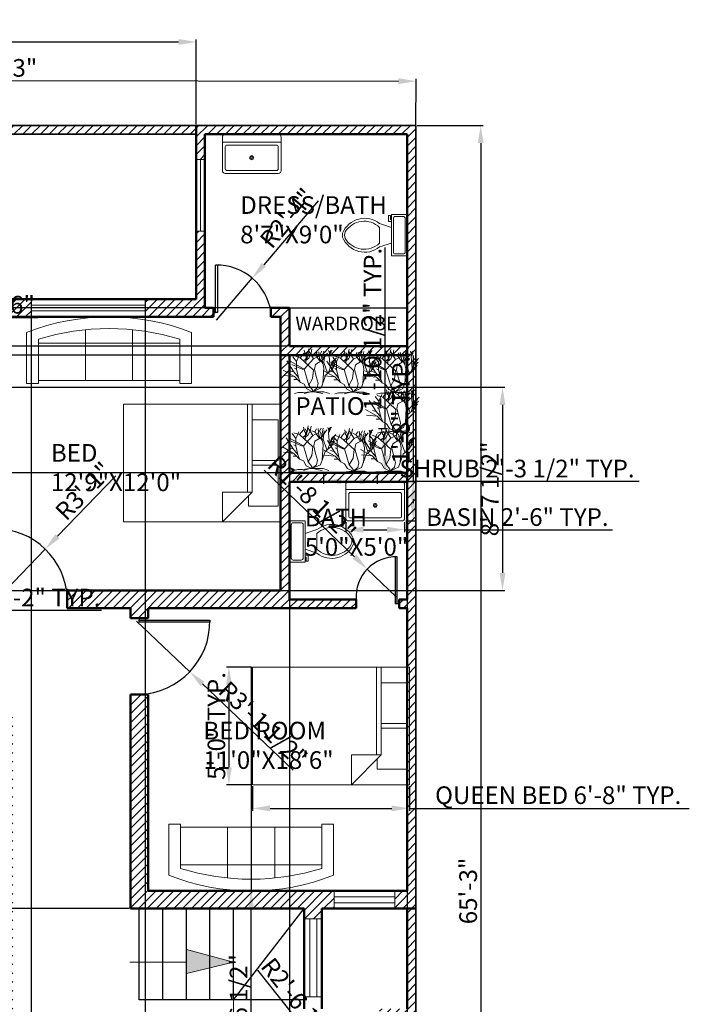
# Model space of a CAD drawing. Units: inches. Extents: x 36184 to 36805, y 18177 to 19069.
# Tile 5 of 5: x 36463 to 36805, y 18560 to 19061. Entities that reach past the tile are written whole.
import ezdxf

# ---------------------------------------------------------------- set-up
doc = ezdxf.new("R2010")
doc.units = ezdxf.units.IN
doc.linetypes.add('ACAD_ISO02W100', pattern=[15, 12, -3])
for name, color, linetype, lineweight in [('A-ANNO-DIMS', 2, 'Continuous', 18), ('A-ANNO-SYMB', 7, 'Continuous', 18), ('A-ANNO-SYMB-PATT', 7, 'Continuous', 13), ('A-AREA-IDEN', 7, 'Continuous', 25), ('A-DOOR', 4, 'Continuous', 25), ('A-FLOR-CASE', 9, 'Continuous', 25), ('A-FLOR-FIXT', 9, 'Continuous', 18), ('A-FLOR-STRS', 7, 'Continuous', 25), ('A-FLOR-STRS-OVHD', 7, 'ACAD_ISO02W100', 18), ('A-FURN', 8, 'Continuous', 18), ('A-GLAZ', 4, 'Continuous', 18), ('A-WALL', 7, 'Continuous', 50), ('C-PROP', 7, 'Continuous', 35), ('L-PLNT', 94, 'Continuous', 13), ('L-SITE-WALL', 7, 'Continuous', 35)]:
    doc.layers.add(name, color=color, linetype=linetype, lineweight=lineweight)
doc.layers.add('A-WALL-PATT', color=244, linetype='Continuous', lineweight=13, true_color=0x991b1e)
doc.styles.get("Standard").update_dxf_attribs({"font": 'arial.ttf'})
doc.dimstyles.new('ISO-25', dxfattribs={"dimtxt": 9, "dimasz": 9, "dimexe": 1.25, "dimexo": 0.625, "dimtad": 1, "dimdec": 1, "dimrnd": 9, "dimlunit": 3, "dimtxsty": 'Standard', "dimcen": 2.5, "dimadec": 0, "dimazin": 0, "dimtfac": 1, "dimtdec": 1, "dimtmove": 0, "dimatfit": 3, "dimfxl": 1, "dimarcsym": 0})

# ---------------------------------------------------------------- blocks, each defined once
blk = doc.blocks.new('Sofa - Roundback 7 ft.')
for p, q in [((-12.00002, -32.4421), (-12.00003, -6.5971)), ((11.99997, -32.4421), (11.99998, -6.5971)), ((-36.000027, -34), (-36.000027, -11.4696)), ((-35.999844, -13.3819), (35.9998, -13.3819)), ((35.99998, -34), (35.99998, -11.4696)), ((-36.000027, -32.4421), (35.99998, -32.4421))]:
    blk.add_line(p, q)
for points in [[(-36.000027, -34), (-42.000027, -34), (-42.000027, -8)], [(41.99998, -8), (41.99998, -34), (35.99998, -34)]]:
    blk.add_lwpolyline(points)
for centre, radius, start, end in [((0, -114.25), 114.25, 68.43141, 111.5686), ((-0.00001, -127.1968), 121.1968, 72.72033, 107.2797)]:
    blk.add_arc(centre, radius, start, end)
blk = doc.blocks.new('Bed - Queen')
for p, q in [((0, -80.00003), (0, 0)), ((0, 0), (59.99999, 0)), ((59.99999, 0), (59.99999, -80.00003)), ((7.99999, -1.2), (28.79998, -1.2)), ((7.99999, -14.4), (7.99999, -1.2)), ((28.79998, -1.2), (28.79998, -14.4)), ((31.19999, -1.2), (51.99999, -1.2)), ((31.19999, -14.4), (31.19999, -1.2)), ((51.99999, -1.2), (51.99999, -16.4)), ((0, -14.4), (44.8, -14.4)), ((59.99999, -29.6), (44.8, -14.4)), ((44.8, -14.4), (44.8, -29.6)), ((44.8, -16.8), (0, -16.8)), ((51.99999, -16.4), (46.79936, -16.4)), ((44.8, -29.6), (59.99999, -29.6)), ((59.99999, -80.00003), (0, -80.00003))]:
    blk.add_line(p, q)
blk = doc.blocks.new('Toilet - top')
for p, q in [((9.5, -6), (9.5, -2)), ((-10, -8.5), (-8, -8.5)), ((-10, -9.5), (-10, -8.5)), ((-7, -9.5), (-10, -9.5)), ((-8, -8.5), (-8, -8)), ((-7, -8), (-7, -9.5)), ((-4, -8), (-6, -14)), ((4, -8), (6, -14)), ((4, -14), (-4, -14))]:
    blk.add_line(p, q)
blk.add_lwpolyline([(10.5, -8), (10.5, 0), (-10.5, 0), (-10.5, -8)], close=True)
for points in [[(-9.5, -2), (-9.5, -6)], [(8.5, -1), (-8.5, -1)], [(-8.5, -7), (8.5, -7)]]:
    blk.add_lwpolyline(points)
for centre, radius, start, end in [((-8.62, -1.88), 0.884, 81.8699, 188.1301), ((8.62, -1.88), 0.884, 351.8699, 98.1301), ((-8.62, -6.12), 0.884, 171.8699, 278.1301), ((8.62, -6.12), 0.884, 261.8699, 8.1301), ((3.52, -21.58), 12.17, 141.4691, 247.9714), ((4.2, -21.82), 11.33, 136.3677, 238.9468), ((-3.52, -21.58), 12.17, 292.0284, 38.5307), ((-4.2, -21.82), 11.33, 301.053, 43.6321), ((0, -27.88), 4, 245.7318, 294.2682), ((0, -29), 4, 254.8605, 285.1395)]:
    blk.add_arc(centre, radius, start, end)
blk = doc.blocks.new('Sink-single - 30 in top')
blk.add_line((-15, -3.999996), (15, -3.999996))
for points in [[(-13.5, 0), (13.5, 0)], [(-15, -18.499996), (-15, -1.5)], [(15, -1.5), (15, -18.499996)], [(-13.5, -17.499996), (-13.5, -6.499996)], [(-12.5, -5.499996), (12.5, -5.499996)], [(13.5, -6.499996), (13.5, -17.499996)], [(13.5, -19.999996), (-13.5, -19.999996)], [(12.5, -18.499996), (-12.5, -18.499996)]]:
    blk.add_lwpolyline(points)
for radius in [1, 0.5]:
    blk.add_circle((0, -11.999996), radius)
for centre, radius, start, end in [((-13.5, -1.5), 1.5, 90, 180), ((13.5, -1.5), 1.5, 0, 90), ((-12.5, -6.499996), 1, 90, 180), ((12.5, -6.499996), 1, 0, 90), ((-13.5, -18.499996), 1.5, 180, 270), ((-12.5, -17.499996), 1, 180, 270), ((12.5, -17.499996), 1, 270, 0), ((13.5, -18.499996), 1.5, 270, 0)]:
    blk.add_arc(centre, radius, start, end)
blk = doc.blocks.new('*D13')
at = {"layer": 'A-ANNO-DIMS', "color": 0, "lineweight": -2, "transparency": 16777216}
for p, q in [((36245.31, 19007.93), (36245.36, 19031.89)), ((36665.31, 19007.11), (36665.36, 19031.07)), ((36254.36, 19030.62), (36656.36, 19029.84))]:
    blk.add_line(p, q, dxfattribs=at)
at = {"layer": 'A-ANNO-DIMS', "color": 0, "transparency": 16777216}
for points in [[(36254.36, 19032.12), (36254.35, 19029.12), (36245.36, 19030.64)], [(36656.36, 19031.34), (36656.35, 19028.34), (36665.36, 19029.82)]]:
    blk.add_solid(points, dxfattribs=at)
at = {"layer": 'Defpoints', "color": 0, "transparency": 16777216}
for p in [(36665.36, 19029.82), (36245.31, 19007.3), (36665.31, 19006.48)]:
    blk.add_point(p, dxfattribs=at)
at = {"layer": 'A-ANNO-DIMS', "color": 0, "transparency": 16777216, "insert": (36455.37, 19035.45), "char_height": 9, "attachment_point": 5, "rotation": 359.8885}
blk.add_mtext('35\'-3"', dxfattribs=at)
blk = doc.blocks.new('*D15')
at = {"layer": 'A-ANNO-DIMS', "color": 0, "lineweight": -2, "transparency": 16777216}
for p, q in [((36665.94, 19007.3), (36699.58, 19007.3)), ((36698.33, 18998.3), (36698.33, 18236.3)), ((36665.94, 18227.3), (36699.58, 18227.3))]:
    blk.add_line(p, q, dxfattribs=at)
at = {"layer": 'A-ANNO-DIMS', "color": 0, "transparency": 16777216}
for points in [[(36696.83, 18998.3), (36699.83, 18998.3), (36698.33, 19007.3)], [(36696.83, 18236.3), (36699.83, 18236.3), (36698.33, 18227.3)]]:
    blk.add_solid(points, dxfattribs=at)
at = {"layer": 'Defpoints', "color": 0, "transparency": 16777216}
for p in [(36665.31, 19007.3), (36665.31, 18227.3), (36698.33, 18227.3)]:
    blk.add_point(p, dxfattribs=at)
at = {"layer": 'A-ANNO-DIMS', "color": 0, "transparency": 16777216, "insert": (36693.1, 18617.3), "char_height": 9, "attachment_point": 5, "rotation": 90}
blk.add_mtext('65\'-3"', dxfattribs=at)
blk = doc.blocks.new('Shrub - elevation')
for p, q in [((-14.88, 18.24), (-12.96, 20.64)), ((-12.471, 19.775), (-12.898, 22.044)), ((-11.28, 19.619), (-12.104, 21.184)), ((-11.921, 18.836), (-10.64, 20.401)), ((-11.433, 18.289), (-10.457, 22.749)), ((-8.16, 17.76), (-10.56, 21.6)), ((-9.48, 19.775), (-8.992, 22.592)), ((-7.2, 19.68), (-8.64, 20.16)), ((-7.2, 19.68), (-6.24, 21.12)), ((-5.086, 17.741), (-5.513, 21.34)), ((-5.28, 19.2), (-3.84, 21.6)), ((-3.84, 16.8), (-0.96, 20.64)), ((-3.377, 18.602), (-2.888, 21.575)), ((-2.88, 15.84), (-2.4, 20.16)), ((-0.508, 21.888), (-0.081, 20.558)), ((-0.203, 19.149), (0.102, 21.34)), ((-0.142, 19.384), (0.59, 20.401)), ((-0.02, 20.01), (0.896, 21.105)), ((0.041, 20.714), (1.384, 22.044)), ((0.102, 21.34), (0.835, 21.888)), ((-18.24, 11.04), (-21.755, 16.655)), ((-12.96, 12.48), (-19.68, 16.32)), ((-16.8, 16.32), (-18.72, 18.72)), ((-14.88, 18.24), (-17.76, 19.2)), ((-16.8, 16.32), (-15.36, 19.68)), ((-16.8, 12.48), (-16.8, 16.32)), ((-8.16, 12), (-14.88, 18.24)), ((-13.325, 16.724), (-11.433, 18.289)), ((-12.96, 12.48), (-8.16, 17.76)), ((-11.677, 19.071), (-12.471, 19.775)), ((-12.043, 15.628), (-11.921, 18.836)), ((-11.982, 16.802), (-10.579, 18.054)), ((-10.579, 18.054), (-9.846, 19.697)), ((-8.16, 17.76), (-5.28, 19.2)), ((-4.8, 16.32), (-7.2, 19.68)), ((-7.2, 14.88), (-3.84, 16.8)), ((-3.377, 15.315), (-5.086, 17.819)), ((-2.88, 12.96), (-4.32, 19.68)), ((-2.766, 16.802), (-3.377, 18.602)), ((-0.96, 10.56), (-2.88, 15.84)), ((0.346, 13.203), (-0.203, 19.149)), ((0.346, 13.203), (1.323, 16.254)), ((0.96, 12), (1.44, 15.36)), ((1.323, 16.254), (3.642, 18.289)), ((1.44, 15.36), (2.88, 17.28)), ((1.92, 13.44), (2.4, 15.36)), ((2.4, 15.36), (3.36, 16.32)), ((-17.76, 8.64), (-23.663, 11.961)), ((-18.24, 11.04), (-20.16, 11.52)), ((-13.92, 12.48), (-19.2, 14.88)), ((-15.84, 8.16), (-18.24, 11.04)), ((-16.8, 12.48), (-17.76, 12.96)), ((-15.84, 8.16), (-16.8, 12.48)), ((-12.96, 12.48), (-13.92, 12.48)), ((-10.56, 4.32), (-12.96, 12.48)), ((-8.64, 7.68), (-8.16, 12)), ((-7.68, 12.48), (-7.2, 14.88)), ((-6.72, 8.64), (-7.68, 12.48)), ((-3.36, 5.28), (-2.88, 12.96)), ((-1.92, 9.6), (0.96, 12)), ((-0.48, 10.8), (0.346, 13.203)), ((0.96, 12), (2.88, 14.88)), ((-17.76, 8.64), (-23.128, 9.222)), ((-16.32, 7.2), (-18.24, 7.2)), ((-14.88, 5.76), (-17.76, 8.64)), ((-14.88, 5.76), (-15.84, 8.16)), ((-12.96, 4.8), (-14.88, 5.76)), ((-10.56, 4.32), (-8.64, 7.68)), ((-5.76, 5.28), (-6.72, 8.64)), ((-6.24, 2.88), (-5.76, 5.28)), ((-4.32, 2.88), (-1.92, 9.6)), ((-15.84, 0.48), (-17.76, 0)), ((-13.44, 0.48), (-15.84, 0.48)), ((-9.6, 0.96), (-13.44, 0.48)), ((-11.52, 2.4), (-12.96, 4.8)), ((-9.6, 0.96), (-12.96, 0)), ((-8.64, 0.96), (-11.52, 2.4)), ((-8.64, 1.92), (-10.56, 4.32)), ((-9.6, 0.96), (-7.68, 0.96)), ((-8.64, 0.96), (-4.32, 2.88)), ((-8.64, 0.96), (-6.24, 2.88)), ((-8.64, 0.96), (-8.64, 1.92)), ((-8.64, 0.96), (-2.88, 0.96)), ((-7.68, 0.96), (-6.24, 0.48)), ((-6.24, 0.48), (-3.36, 0)), ((-2.88, 0.96), (0, 0))]:
    blk.add_line(p, q)
blk = doc.blocks.new('DOOR-LEAF-24IN')
for p, q in [((1, 0), (1, 24)), ((1, 24), (2, 24)), ((2, 24), (2, 0)), ((0, 0), (1, 0)), ((1, 0), (2, 0))]:
    blk.add_line(p, q)
blk = doc.blocks.new('DOOR-LEAF-36IN')
for p, q in [((1, 36), (0, 36)), ((0, 36), (0, 0)), ((1, 0), (1, 36)), ((0, 0), (1, 0)), ((2, 0), (1, 0))]:
    blk.add_line(p, q)
blk = doc.blocks.new('*D24')
at = {"layer": 'A-ANNO-DIMS', "color": 0, "lineweight": -2, "transparency": 16777216}
for p, q in [((36618.26, 18829.49), (36618.26, 18824.77)), ((36627.26, 18826.02), (36636.57, 18826.02)), ((36645.57, 18829.49), (36645.57, 18824.77)), ((36645.57, 18826.02), (36779.11, 18826.02))]:
    blk.add_line(p, q, dxfattribs=at)
at = {"layer": 'A-ANNO-DIMS', "color": 0, "transparency": 16777216}
for points in [[(36627.26, 18827.52), (36627.26, 18824.52), (36618.26, 18826.02)], [(36636.57, 18827.52), (36636.57, 18824.52), (36645.57, 18826.02)]]:
    blk.add_solid(points, dxfattribs=at)
at = {"layer": 'Defpoints', "color": 0, "transparency": 16777216}
for p in [(36618.26, 18830.12), (36645.57, 18830.12), (36645.57, 18826.02)]:
    blk.add_point(p, dxfattribs=at)
at = {"layer": 'A-ANNO-DIMS', "color": 0, "transparency": 16777216, "insert": (36716.84, 18831.31), "char_height": 9, "attachment_point": 5}
blk.add_mtext('SHRUB 2\'-3 1/2" TYP.', dxfattribs=at)
blk = doc.blocks.new('*D25')
at = {"layer": 'A-ANNO-DIMS', "color": 0, "lineweight": -2, "transparency": 16777216}
for p, q in [((36649.66, 18852.87), (36649.66, 18945.1)), ((36646.19, 18852.87), (36650.91, 18852.87)), ((36649.66, 18839.12), (36649.66, 18843.87)), ((36646.19, 18830.12), (36650.91, 18830.12))]:
    blk.add_line(p, q, dxfattribs=at)
at = {"layer": 'A-ANNO-DIMS', "color": 0, "transparency": 16777216}
for points in [[(36648.16, 18843.87), (36651.16, 18843.87), (36649.66, 18852.87)], [(36648.16, 18839.12), (36651.16, 18839.12), (36649.66, 18830.12)]]:
    blk.add_solid(points, dxfattribs=at)
at = {"layer": 'Defpoints', "color": 0, "transparency": 16777216}
for p in [(36645.57, 18852.87), (36649.66, 18852.87), (36645.57, 18830.12)]:
    blk.add_point(p, dxfattribs=at)
at = {"layer": 'A-ANNO-DIMS', "color": 0, "transparency": 16777216, "insert": (36644.38, 18903.48), "char_height": 9, "attachment_point": 5, "rotation": 90}
blk.add_mtext('1\'-10 1/2" TYP.', dxfattribs=at)
blk = doc.blocks.new('*D29')
at = {"layer": 'A-ANNO-DIMS', "color": 0, "lineweight": -2, "transparency": 16777216}
for p, q in [((36429, 18765.18), (36429, 18759.15)), ((36431, 18765.18), (36431, 18759.15)), ((36420, 18760.4), (36411, 18760.4)), ((36429, 18760.4), (36431, 18760.4)), ((36440, 18760.4), (36505.11, 18760.4))]:
    blk.add_line(p, q, dxfattribs=at)
at = {"layer": 'A-ANNO-DIMS', "color": 0, "transparency": 16777216}
for points in [[(36420, 18761.9), (36420, 18758.9), (36429, 18760.4)], [(36440, 18761.9), (36440, 18758.9), (36431, 18760.4)]]:
    blk.add_solid(points, dxfattribs=at)
at = {"layer": 'Defpoints', "color": 0, "transparency": 16777216}
for p in [(36429, 18765.8), (36431, 18765.8), (36431, 18760.4)]:
    blk.add_point(p, dxfattribs=at)
at = {"layer": 'A-ANNO-DIMS', "color": 0, "transparency": 16777216, "insert": (36477.06, 18765.62), "char_height": 9, "attachment_point": 5}
blk.add_mtext('0\'-2" TYP.', dxfattribs=at)
blk = doc.blocks.new('*D30')
at = {"layer": 'A-ANNO-DIMS', "color": 0, "lineweight": -2, "transparency": 16777216}
for p, q in [((36582.01, 18670.73), (36582.01, 18658.11)), ((36662.01, 18670.73), (36662.01, 18658.11)), ((36591.01, 18659.36), (36653.01, 18659.36)), ((36662.01, 18659.36), (36804.65, 18659.36))]:
    blk.add_line(p, q, dxfattribs=at)
at = {"layer": 'A-ANNO-DIMS', "color": 0, "transparency": 16777216}
for points in [[(36591.01, 18660.86), (36591.01, 18657.86), (36582.01, 18659.36)], [(36653.01, 18660.86), (36653.01, 18657.86), (36662.01, 18659.36)]]:
    blk.add_solid(points, dxfattribs=at)
at = {"layer": 'Defpoints', "color": 0, "transparency": 16777216}
for p in [(36582.01, 18671.36), (36662.01, 18671.36), (36662.01, 18659.36)]:
    blk.add_point(p, dxfattribs=at)
at = {"layer": 'A-ANNO-DIMS', "color": 0, "transparency": 16777216, "insert": (36737.83, 18664.91), "char_height": 9, "attachment_point": 5}
blk.add_mtext('QUEEN BED 6\'-8" TYP.', dxfattribs=at)
blk = doc.blocks.new('*D31')
at = {"layer": 'A-ANNO-DIMS', "color": 0, "lineweight": -2, "transparency": 16777216}
for p, q in [((36581.39, 18731.36), (36568.76, 18731.36)), ((36570.01, 18722.36), (36570.01, 18680.36)), ((36581.39, 18671.36), (36568.76, 18671.36))]:
    blk.add_line(p, q, dxfattribs=at)
at = {"layer": 'A-ANNO-DIMS', "color": 0, "transparency": 16777216}
for points in [[(36568.51, 18722.36), (36571.51, 18722.36), (36570.01, 18731.36)], [(36568.51, 18680.36), (36571.51, 18680.36), (36570.01, 18671.36)]]:
    blk.add_solid(points, dxfattribs=at)
at = {"layer": 'Defpoints', "color": 0, "transparency": 16777216}
for p in [(36582.01, 18731.36), (36570.01, 18671.36), (36582.01, 18671.36)]:
    blk.add_point(p, dxfattribs=at)
at = {"layer": 'A-ANNO-DIMS', "color": 0, "transparency": 16777216, "insert": (36564.79, 18701.36), "char_height": 9, "attachment_point": 5, "rotation": 90}
blk.add_mtext('5\'-0" TYP.', dxfattribs=at)
blk = doc.blocks.new('*D34')
at = {"layer": 'A-ANNO-DIMS', "color": 0, "lineweight": -2, "transparency": 16777216}
for p, q in [((36629.54, 18805.19), (36629.54, 18800.07)), ((36659.54, 18805.19), (36659.54, 18800.07)), ((36638.54, 18801.32), (36650.54, 18801.32)), ((36659.54, 18801.32), (36765.47, 18801.32))]:
    blk.add_line(p, q, dxfattribs=at)
at = {"layer": 'A-ANNO-DIMS', "color": 0, "transparency": 16777216}
for points in [[(36638.54, 18802.82), (36638.54, 18799.82), (36629.54, 18801.32)], [(36650.54, 18802.82), (36650.54, 18799.82), (36659.54, 18801.32)]]:
    blk.add_solid(points, dxfattribs=at)
at = {"layer": 'Defpoints', "color": 0, "transparency": 16777216}
for p in [(36629.54, 18805.82), (36659.54, 18805.82), (36659.54, 18801.32)]:
    blk.add_point(p, dxfattribs=at)
at = {"layer": 'A-ANNO-DIMS', "color": 0, "transparency": 16777216, "insert": (36717, 18806.6), "char_height": 9, "attachment_point": 5}
blk.add_mtext('BASIN 2\'-6" TYP.', dxfattribs=at)
blk = doc.blocks.new('*D35')
at = {"layer": 'A-ANNO-DIMS', "color": 0, "lineweight": -2, "transparency": 16777216}
for p, q in [((36664.04, 18825.82), (36664.04, 18890.08)), ((36660.16, 18825.82), (36665.29, 18825.82)), ((36664.04, 18814.82), (36664.04, 18816.82)), ((36660.16, 18805.82), (36665.29, 18805.82))]:
    blk.add_line(p, q, dxfattribs=at)
at = {"layer": 'A-ANNO-DIMS', "color": 0, "transparency": 16777216}
for points in [[(36662.54, 18816.82), (36665.54, 18816.82), (36664.04, 18825.82)], [(36662.54, 18814.82), (36665.54, 18814.82), (36664.04, 18805.82)]]:
    blk.add_solid(points, dxfattribs=at)
at = {"layer": 'Defpoints', "color": 0, "transparency": 16777216}
for p in [(36659.54, 18825.82), (36664.04, 18825.82), (36659.54, 18805.82)]:
    blk.add_point(p, dxfattribs=at)
at = {"layer": 'A-ANNO-DIMS', "color": 0, "transparency": 16777216, "insert": (36658.82, 18862.45), "char_height": 9, "attachment_point": 5, "rotation": 90}
blk.add_mtext('1\'-8" TYP.', dxfattribs=at)
blk = doc.blocks.new('*D40')
at = {"layer": 'A-ANNO-DIMS', "color": 0, "lineweight": -2, "transparency": 16777216}
for p, q in [((36360.76, 18905.62), (36360.76, 18910.74)), ((36390.76, 18905.62), (36390.76, 18910.74)), ((36369.76, 18909.49), (36381.76, 18909.49)), ((36390.76, 18909.49), (36472.67, 18909.49))]:
    blk.add_line(p, q, dxfattribs=at)
at = {"layer": 'A-ANNO-DIMS', "color": 0, "transparency": 16777216}
for points in [[(36369.76, 18910.99), (36369.76, 18907.99), (36360.76, 18909.49)], [(36381.76, 18910.99), (36381.76, 18907.99), (36390.76, 18909.49)]]:
    blk.add_solid(points, dxfattribs=at)
at = {"layer": 'Defpoints', "color": 0, "transparency": 16777216}
for p in [(36390.76, 18909.49), (36360.76, 18904.99), (36390.76, 18904.99)]:
    blk.add_point(p, dxfattribs=at)
at = {"layer": 'A-ANNO-DIMS', "color": 0, "transparency": 16777216, "insert": (36436.22, 18914.77), "char_height": 9, "attachment_point": 5}
blk.add_mtext('RANGE 2\'-6"', dxfattribs=at)
blk = doc.blocks.new('*D45')
at = {"layer": 'A-ANNO-DIMS', "color": 0, "lineweight": -2, "transparency": 16777216}
for p, q in [((36245.31, 19007.93), (36245.31, 19051.05)), ((36553.31, 19007.93), (36553.31, 19051.05)), ((36254.31, 19049.8), (36544.31, 19049.8))]:
    blk.add_line(p, q, dxfattribs=at)
at = {"layer": 'A-ANNO-DIMS', "color": 0, "transparency": 16777216}
for points in [[(36254.31, 19051.3), (36254.31, 19048.3), (36245.31, 19049.8)], [(36544.31, 19051.3), (36544.31, 19048.3), (36553.31, 19049.8)]]:
    blk.add_solid(points, dxfattribs=at)
at = {"layer": 'Defpoints', "color": 0, "transparency": 16777216}
for p in [(36553.31, 19049.8), (36245.31, 19007.3), (36553.31, 19007.3)]:
    blk.add_point(p, dxfattribs=at)
at = {"layer": 'A-ANNO-DIMS', "color": 0, "transparency": 16777216, "insert": (36399.31, 19055.02), "char_height": 9, "attachment_point": 5}
blk.add_mtext('25\'-8"', dxfattribs=at)
blk = doc.blocks.new('*D47')
at = {"layer": 'A-ANNO-DIMS', "color": 0, "lineweight": -2, "transparency": 16777216}
for p, q in [((36519.19, 18608.3), (36201.56, 18608.3)), ((36202.81, 18518.3), (36202.81, 18599.3)), ((36519.19, 18509.3), (36201.56, 18509.3))]:
    blk.add_line(p, q, dxfattribs=at)
at = {"layer": 'A-ANNO-DIMS', "color": 0, "transparency": 16777216}
for points in [[(36201.31, 18599.3), (36204.31, 18599.3), (36202.81, 18608.3)], [(36201.31, 18518.3), (36204.31, 18518.3), (36202.81, 18509.3)]]:
    blk.add_solid(points, dxfattribs=at)
at = {"layer": 'Defpoints', "color": 0, "transparency": 16777216}
for p in [(36202.81, 18608.3), (36519.81, 18608.3), (36519.81, 18509.3)]:
    blk.add_point(p, dxfattribs=at)
at = {"layer": 'A-ANNO-DIMS', "color": 0, "transparency": 16777216, "insert": (36197.59, 18558.8), "char_height": 9, "attachment_point": 5, "rotation": 90}
blk.add_mtext('8\'-3"', dxfattribs=at)
blk = doc.blocks.new('*D48')
at = {"layer": 'A-ANNO-DIMS', "color": 0, "lineweight": -2, "transparency": 16777216}
for p, q in [((36600.81, 18829.68), (36600.81, 18183.55)), ((36660.81, 18829.68), (36660.81, 18183.55)), ((36609.81, 18184.8), (36651.81, 18184.8))]:
    blk.add_line(p, q, dxfattribs=at)
at = {"layer": 'A-ANNO-DIMS', "color": 0, "transparency": 16777216}
for points in [[(36609.81, 18186.3), (36609.81, 18183.3), (36600.81, 18184.8)], [(36651.81, 18186.3), (36651.81, 18183.3), (36660.81, 18184.8)]]:
    blk.add_solid(points, dxfattribs=at)
at = {"layer": 'Defpoints', "color": 0, "transparency": 16777216}
for p in [(36600.81, 18830.3), (36660.81, 18830.3), (36660.81, 18184.8)]:
    blk.add_point(p, dxfattribs=at)
at = {"layer": 'A-ANNO-DIMS', "color": 0, "transparency": 16777216, "insert": (36630.81, 18190.02), "char_height": 9, "attachment_point": 5}
blk.add_mtext('5\'-0"', dxfattribs=at)
blk = doc.blocks.new('*D49')
at = {"layer": 'A-ANNO-DIMS', "color": 0, "lineweight": -2, "transparency": 16777216}
for p, q in [((36600.19, 18890.3), (36201.56, 18890.3)), ((36202.81, 18839.3), (36202.81, 18881.3)), ((36600.19, 18830.3), (36201.56, 18830.3))]:
    blk.add_line(p, q, dxfattribs=at)
at = {"layer": 'A-ANNO-DIMS', "color": 0, "transparency": 16777216}
for points in [[(36201.31, 18881.3), (36204.31, 18881.3), (36202.81, 18890.3)], [(36201.31, 18839.3), (36204.31, 18839.3), (36202.81, 18830.3)]]:
    blk.add_solid(points, dxfattribs=at)
at = {"layer": 'Defpoints', "color": 0, "transparency": 16777216}
for p in [(36202.81, 18890.3), (36600.81, 18890.3), (36600.81, 18830.3)]:
    blk.add_point(p, dxfattribs=at)
at = {"layer": 'A-ANNO-DIMS', "color": 0, "transparency": 16777216, "insert": (36197.59, 18860.3), "char_height": 9, "attachment_point": 5, "rotation": 90}
blk.add_mtext('5\'-0"', dxfattribs=at)
blk = doc.blocks.new('*D50')
at = {"layer": 'A-ANNO-DIMS', "color": 0, "lineweight": -2, "transparency": 16777216}
for p, q in [((36202.81, 18914.3), (36202.81, 18968.6)), ((36600.19, 18914.3), (36201.56, 18914.3)), ((36202.81, 18903.8), (36202.81, 18905.3)), ((36600.19, 18894.8), (36201.56, 18894.8))]:
    blk.add_line(p, q, dxfattribs=at)
at = {"layer": 'A-ANNO-DIMS', "color": 0, "transparency": 16777216}
for points in [[(36201.31, 18905.3), (36204.31, 18905.3), (36202.81, 18914.3)], [(36201.31, 18903.8), (36204.31, 18903.8), (36202.81, 18894.8)]]:
    blk.add_solid(points, dxfattribs=at)
at = {"layer": 'Defpoints', "color": 0, "transparency": 16777216}
for p in [(36202.81, 18914.3), (36600.81, 18914.3), (36600.81, 18894.8)]:
    blk.add_point(p, dxfattribs=at)
at = {"layer": 'A-ANNO-DIMS', "color": 0, "transparency": 16777216, "insert": (36197.53, 18945.95), "char_height": 9, "attachment_point": 5, "rotation": 90}
blk.add_mtext('1\'-7 1/2"', dxfattribs=at)
blk = doc.blocks.new('*D56')
at = {"layer": 'A-ANNO-DIMS', "color": 0, "lineweight": -2, "transparency": 16777216}
for p, q in [((36355.59, 18873.92), (36710.68, 18873.92)), ((36709.43, 18864.92), (36709.43, 18779.3)), ((36355.59, 18770.3), (36710.68, 18770.3))]:
    blk.add_line(p, q, dxfattribs=at)
at = {"layer": 'A-ANNO-DIMS', "color": 0, "transparency": 16777216}
for points in [[(36707.93, 18864.92), (36710.93, 18864.92), (36709.43, 18873.92)], [(36707.93, 18779.3), (36710.93, 18779.3), (36709.43, 18770.3)]]:
    blk.add_solid(points, dxfattribs=at)
at = {"layer": 'Defpoints', "color": 0, "transparency": 16777216}
for p in [(36354.96, 18873.92), (36354.96, 18770.3), (36709.43, 18770.3)]:
    blk.add_point(p, dxfattribs=at)
at = {"layer": 'A-ANNO-DIMS', "color": 0, "transparency": 16777216, "insert": (36704.15, 18822.11), "char_height": 9, "attachment_point": 5, "rotation": 90}
blk.add_mtext('8\'-7 1/2"', dxfattribs=at)
blk = doc.blocks.new('*D59')
at = {"layer": 'A-ANNO-DIMS', "color": 0, "lineweight": -2, "transparency": 16777216}
for p, q in [((36469.15, 18918.18), (36469.15, 18183.55)), ((36527.35, 18918.18), (36527.35, 18183.55)), ((36478.15, 18184.8), (36518.35, 18184.8))]:
    blk.add_line(p, q, dxfattribs=at)
at = {"layer": 'A-ANNO-DIMS', "color": 0, "transparency": 16777216}
for points in [[(36478.15, 18186.3), (36478.15, 18183.3), (36469.15, 18184.8)], [(36518.35, 18186.3), (36518.35, 18183.3), (36527.35, 18184.8)]]:
    blk.add_solid(points, dxfattribs=at)
at = {"layer": 'Defpoints', "color": 0, "transparency": 16777216}
for p in [(36469.15, 18918.8), (36527.35, 18918.8), (36527.35, 18184.8)]:
    blk.add_point(p, dxfattribs=at)
at = {"layer": 'A-ANNO-DIMS', "color": 0, "transparency": 16777216, "insert": (36498.25, 18190.02), "char_height": 9, "attachment_point": 5}
blk.add_mtext('4\'-10"', dxfattribs=at)
blk = doc.blocks.new('*D63')
at = {"layer": 'A-ANNO-DIMS', "color": 0, "lineweight": -2, "transparency": 16777216}
for p, q in [((36522.91, 18754.76), (36550.02, 18728.99)), ((36602.76, 18678.87), (36556.55, 18722.79))]:
    blk.add_line(p, q, dxfattribs=at)
at = {"layer": 'A-ANNO-DIMS', "color": 0, "transparency": 16777216}
blk.add_solid([(36557.58, 18723.88), (36555.51, 18721.7), (36550.02, 18728.99)], dxfattribs=at)
at = {"layer": 'Defpoints', "color": 0, "transparency": 16777216}
for p in [(36522.91, 18754.76), (36550.02, 18728.99)]:
    blk.add_point(p, dxfattribs=at)
at = {"layer": 'A-ANNO-DIMS', "color": 0, "transparency": 16777216, "insert": (36586.56, 18701.56), "char_height": 9, "attachment_point": 5, "rotation": 316.4568}
blk.add_mtext('R3\'-1 1/2"', dxfattribs=at)
blk = doc.blocks.new('*D64')
at = {"layer": 'A-ANNO-DIMS', "color": 0, "lineweight": -2, "transparency": 16777216}
for p, q in [((36512.31, 18828.76), (36482.61, 18797.96)), ((36450.79, 18764.96), (36476.36, 18791.48))]:
    blk.add_line(p, q, dxfattribs=at)
at = {"layer": 'A-ANNO-DIMS', "color": 0, "transparency": 16777216}
blk.add_solid([(36481.53, 18799), (36483.69, 18796.92), (36476.36, 18791.48)], dxfattribs=at)
at = {"layer": 'Defpoints', "color": 0, "transparency": 16777216}
for p in [(36476.36, 18791.48), (36450.79, 18764.96)]:
    blk.add_point(p, dxfattribs=at)
at = {"layer": 'A-ANNO-DIMS', "color": 0, "transparency": 16777216, "insert": (36496.82, 18820.23), "char_height": 9, "attachment_point": 5, "rotation": 46.0444}
blk.add_mtext('R3\'-1"', dxfattribs=at)
blk = doc.blocks.new('*D65')
at = {"layer": 'A-ANNO-DIMS', "color": 0, "lineweight": -2, "transparency": 16777216}
for p, q in [((36584.61, 18576.97), (36624.23, 18527.01)), ((36648.74, 18496.11), (36629.82, 18519.96))]:
    blk.add_line(p, q, dxfattribs=at)
at = {"layer": 'A-ANNO-DIMS', "color": 0, "transparency": 16777216}
blk.add_solid([(36625.4, 18527.95), (36623.05, 18526.08), (36629.82, 18519.96)], dxfattribs=at)
at = {"layer": 'Defpoints', "color": 0, "transparency": 16777216}
for p in [(36629.82, 18519.96), (36648.74, 18496.11)]:
    blk.add_point(p, dxfattribs=at)
at = {"layer": 'A-ANNO-DIMS', "color": 0, "transparency": 16777216, "insert": (36605.76, 18558.8), "char_height": 9, "attachment_point": 5, "rotation": 308.4188}
blk.add_mtext('R2\'-6 1/2"', dxfattribs=at)
blk = doc.blocks.new('*D66')
at = {"layer": 'A-ANNO-DIMS', "color": 0, "lineweight": -2, "transparency": 16777216}
for p, q in [((36615.51, 18968.82), (36587.73, 18936.28)), ((36563.69, 18908.13), (36581.88, 18929.43))]:
    blk.add_line(p, q, dxfattribs=at)
at = {"layer": 'A-ANNO-DIMS', "color": 0, "transparency": 16777216}
blk.add_solid([(36586.59, 18937.25), (36588.87, 18935.31), (36581.88, 18929.43)], dxfattribs=at)
at = {"layer": 'Defpoints', "color": 0, "transparency": 16777216}
for p in [(36581.88, 18929.43), (36563.69, 18908.13)]:
    blk.add_point(p, dxfattribs=at)
at = {"layer": 'A-ANNO-DIMS', "color": 0, "transparency": 16777216, "insert": (36600.63, 18959.31), "char_height": 9, "attachment_point": 5, "rotation": 49.5079}
blk.add_mtext('R2\'-4"', dxfattribs=at)
blk = doc.blocks.new('*D71')
at = {"layer": 'A-ANNO-DIMS', "color": 0, "lineweight": -2, "transparency": 16777216}
for p, q in [((36581.36, 18731.55), (36581.36, 18617.3)), ((36581.36, 18511.74), (36581.36, 18608.3))]:
    blk.add_line(p, q, dxfattribs=at)
at = {"layer": 'A-ANNO-DIMS', "color": 0, "transparency": 16777216}
blk.add_solid([(36579.86, 18608.3), (36582.86, 18608.3), (36581.36, 18617.3)], dxfattribs=at)
at = {"layer": 'Defpoints', "color": 0, "transparency": 16777216}
for p in [(36581.36, 18731.55), (36581.36, 18617.3)]:
    blk.add_point(p, dxfattribs=at)
at = {"layer": 'A-ANNO-DIMS', "color": 0, "transparency": 16777216, "insert": (36576.08, 18548.75), "char_height": 9, "attachment_point": 5, "rotation": 90}
blk.add_mtext('7X R9\'-6 1/2"', dxfattribs=at)
blk = doc.blocks.new('*D74')
at = {"layer": 'A-ANNO-DIMS', "color": 0, "lineweight": -2, "transparency": 16777216}
for p, q in [((36588.04, 18831.72), (36634, 18787.52)), ((36655.23, 18767.1), (36640.48, 18781.28))]:
    blk.add_line(p, q, dxfattribs=at)
at = {"layer": 'A-ANNO-DIMS', "color": 0, "transparency": 16777216}
blk.add_solid([(36635.04, 18788.6), (36632.96, 18786.44), (36640.48, 18781.28)], dxfattribs=at)
at = {"layer": 'Defpoints', "color": 0, "transparency": 16777216}
for p in [(36640.48, 18781.28), (36655.23, 18767.1)]:
    blk.add_point(p, dxfattribs=at)
at = {"layer": 'A-ANNO-DIMS', "color": 0, "transparency": 16777216, "insert": (36611.43, 18816.54), "char_height": 9, "attachment_point": 5, "rotation": 316.1185}
blk.add_mtext('R1\'-8 1/2"', dxfattribs=at)

msp = doc.modelspace()

# ---------------------------------------------------------------- hatches: boundary and pattern name
at = {"layer": 'A-ANNO-SYMB-PATT'}
h = msp.add_hatch(color=256, dxfattribs=at)
h.dxf.hatch_style = 1
h.paths.add_polyline_path([(36560.31, 18584.19), (36548.31, 18587.4), (36548.31, 18575.21), (36560.31, 18578.09)])
h.paths.add_polyline_path([(36572.31, 18580.97), (36560.31, 18584.19), (36560.31, 18578.09)])
at = {"layer": 'A-WALL-PATT'}
h = msp.add_hatch(dxfattribs=at)
h.set_pattern_fill('ANSI31', color=256)
h.paths.add_polyline_path([(36318.81, 18555.8), (36459.81, 18555.8), (36459.81, 18705.8), (36440.41, 18705.8), (36440.41, 18696.8), (36450.81, 18696.8), (36450.81, 18564.8), (36318.81, 18564.8), (36318.81, 18591.83), (36309.81, 18591.83), (36309.81, 18525.65), (36318.81, 18525.65)], flags=17)
h.paths.add_polyline_path([(36318.81, 18455.41), (36309.81, 18455.41), (36309.81, 18402.8), (36338.76, 18402.8), (36338.76, 18411.8), (36318.81, 18411.8)], flags=17)
h.paths.add_polyline_path([(36423.09, 18411.8), (36400.25, 18411.8), (36400.25, 18402.8), (36423.09, 18402.8)], flags=17)
h.paths.add_polyline_path([(36492.81, 18478.27), (36496.58, 18481.34), (36494.6, 18487.78), (36492.81, 18486.25), (36483.81, 18479.84), (36483.81, 18411.8), (36473.38, 18411.8), (36473.38, 18402.8), (36483.81, 18402.8), (36483.81, 18356.3), (36483.81, 18347.3), (36519.81, 18347.3), (36524.04, 18347.3), (36524.04, 18356.3), (36492.81, 18356.3)], flags=17)
h.paths.add_polyline_path([(36665.31, 18608.3), (36660.81, 18608.3), (36660.81, 18557.3), (36646.76, 18557.3), (36646.76, 18552.8), (36660.81, 18552.8), (36660.81, 18504.8), (36650.24, 18504.8), (36650.24, 18500.3), (36660.81, 18500.3), (36660.81, 18356.3), (36622.58, 18356.3), (36622.58, 18347.3), (36665.31, 18347.3)])
h.paths.add_polyline_path([(36608.31, 18509.3), (36519.81, 18509.3), (36513.55, 18503.95), (36517.84, 18498.69), (36519.81, 18500.3), (36608.31, 18500.3)])
h.paths.add_polyline_path([(36254.31, 18411.79), (36249.81, 18411.79), (36249.81, 19002.8), (36553.31, 19002.8), (36553.31, 19007.3), (36245.31, 19007.3), (36245.31, 18288.82), (36254.31, 18288.82)])
h.paths.add_polyline_path([(36342.97, 18918.8), (36309.81, 18918.8), (36309.81, 18747.12), (36314.31, 18747.12), (36314.31, 18765.8), (36384.81, 18765.8), (36384.81, 18701.3), (36350.57, 18701.3), (36350.57, 18696.8), (36396.53, 18696.8), (36396.53, 18705.8), (36389.31, 18705.8), (36389.31, 18761.3), (36393.31, 18761.3), (36393.31, 18770.3), (36384.81, 18770.3), (36318.81, 18770.3), (36318.81, 18909.8), (36342.97, 18909.8)], flags=17)
h.paths.add_polyline_path([(36469.15, 18918.8), (36403.35, 18918.8), (36403.35, 18909.8), (36434.31, 18909.8), (36434.31, 18770.3), (36431, 18770.3), (36431, 18761.3), (36449.29, 18761.3), (36449.29, 18770.3), (36443.31, 18770.3), (36443.31, 18909.8), (36469.15, 18909.8)], flags=17)
h.paths.add_polyline_path([(36557.81, 18953.44), (36553.31, 18953.44), (36553.31, 18918.8), (36527.35, 18918.8), (36527.35, 18909.8), (36553.31, 18909.8), (36562.16, 18909.8), (36562.16, 18914.3), (36557.81, 18914.3)])
h.paths.add_polyline_path([(36665.31, 19007.3), (36553.31, 19007.3), (36553.31, 19002.8), (36553.31, 18989.93), (36557.81, 18989.93), (36557.81, 19002.8), (36660.81, 19002.8), (36660.81, 18765.8), (36656.73, 18765.8), (36656.73, 18761.3), (36660.81, 18761.3), (36660.81, 18617.3), (36654.49, 18617.3), (36654.49, 18608.3), (36665.31, 18608.3)])
h.paths.add_polyline_path([(36600.81, 18890.3), (36596.31, 18890.3), (36596.31, 18770.3), (36487.63, 18770.3), (36487.63, 18761.3), (36519.81, 18761.3), (36519.81, 18756.26), (36528.81, 18756.26), (36528.81, 18761.3), (36634.81, 18761.3), (36634.81, 18765.8), (36600.81, 18765.8), (36600.81, 18825.8), (36660.81, 18825.8), (36660.81, 18830.3), (36600.81, 18830.3)])
h.paths.add_polyline_path([(36600.81, 18914.3), (36596.31, 18914.3), (36591.43, 18914.3), (36591.43, 18909.8), (36596.31, 18909.8), (36596.31, 18890.3), (36660.81, 18890.3), (36660.81, 18894.8), (36600.81, 18894.8)], flags=17)
h.paths.add_polyline_path([(36623.57, 18617.3), (36528.81, 18617.3), (36528.81, 18717.38), (36519.81, 18717.38), (36519.81, 18608.3), (36608.31, 18608.3), (36608.31, 18603.13), (36617.31, 18603.13), (36617.31, 18608.3), (36623.57, 18608.3)])
h.paths.add_polyline_path([(36602.02, 18898.95), (36663.11, 18898.95), (36663.11, 18913.37), (36602.02, 18913.37)], flags=25)

# ---------------------------------------------------------------- linework, layer by layer
at = {"layer": 'A-ANNO-SYMB'}
for p, q in [((36548.31, 18575.21), (36548.31, 18587.4)), ((36548.31, 18587.4), (36572.31, 18580.97)), ((36519.56, 18580.97), (36548.31, 18580.97)), ((36572.31, 18580.97), (36548.31, 18575.21))]:
    msp.add_line(p, q, dxfattribs=at)
at = {"layer": 'A-DOOR'}
for p, q in [((36563.16, 18912.05), (36563.16, 18936.14)), ((36564.16, 18936.14), (36563.16, 18936.14)), ((36564.16, 18936.14), (36564.16, 18912.05)), ((36562.16, 18912.05), (36563.16, 18912.05)), ((36564.16, 18912.05), (36563.16, 18912.05))]:
    msp.add_line(p, q, dxfattribs=at)
for centre, radius, start, end in [((36563.69, 18908.13), 28.02, 8.0553, 90.9608), ((36450.79, 18764.96), 36.85, 1.3121, 90.7775), ((36655.23, 18767.1), 20.46, 88.5995, 183.6381), ((36522.91, 18754.76), 37.41, 272.1482, 0.7659)]:
    msp.add_arc(centre, radius, start, end, dxfattribs=at)
at = {"layer": 'A-FLOR-CASE'}
msp.add_line((36600.81, 18914.3), (36660.81, 18914.3), dxfattribs=at)
at = {"layer": 'A-FLOR-STRS'}
for p, q in [((36524.31, 18561.8), (36524.31, 18608.3)), ((36536.31, 18561.8), (36536.31, 18608.3)), ((36548.31, 18561.8), (36548.31, 18608.3)), ((36560.31, 18561.8), (36560.31, 18608.3)), ((36572.31, 18561.8), (36572.31, 18608.3)), ((36572.31, 18561.8), (36608.31, 18608.3)), ((36608.31, 18561.8), (36524.31, 18561.8))]:
    msp.add_line(p, q, dxfattribs=at)
at = {"layer": 'A-FLOR-STRS-OVHD'}
msp.add_line((36572.31, 18552.8), (36572.31, 18561.8), dxfattribs=at)
at = {"layer": 'A-GLAZ'}
for p, q in [((36557.81, 18989.93), (36553.31, 18989.93)), ((36555.56, 18989.93), (36555.56, 18953.44)), ((36557.81, 18953.44), (36553.31, 18953.44)), ((36469.15, 18918.8), (36469.15, 18909.8)), ((36527.35, 18915.8), (36469.15, 18915.8)), ((36527.35, 18918.8), (36527.35, 18909.8)), ((36527.35, 18912.8), (36469.15, 18912.8)), ((36623.57, 18617.3), (36623.57, 18608.3)), ((36654.49, 18617.3), (36654.49, 18608.3)), ((36654.49, 18614.3), (36623.57, 18614.3)), ((36654.49, 18611.3), (36623.57, 18611.3)), ((36617.31, 18603.13), (36608.31, 18603.13)), ((36611.18, 18603.13), (36611.18, 18563.28)), ((36614.84, 18603.13), (36614.84, 18563.28)), ((36617.31, 18563.28), (36608.31, 18563.28))]:
    msp.add_line(p, q, dxfattribs=at)
at = {"layer": 'A-WALL'}
for p, q in [((36553.31, 18918.8), (36553.31, 19007.3)), ((36660.81, 19002.8), (36557.81, 19002.8)), ((36557.81, 18914.3), (36557.81, 19002.8)), ((36660.81, 18765.8), (36660.81, 19002.8)), ((36553.31, 18918.8), (36309.81, 18918.8)), ((36557.81, 18914.3), (36562.16, 18914.3)), ((36562.16, 18914.3), (36562.16, 18909.8)), ((36591.43, 18914.3), (36591.43, 18909.8)), ((36591.43, 18914.3), (36596.31, 18914.3)), ((36596.31, 18914.3), (36600.81, 18914.3)), ((36600.81, 18894.8), (36600.81, 18914.3)), ((36553.31, 18909.8), (36443.31, 18909.8)), ((36553.31, 18909.8), (36562.16, 18909.8)), ((36591.43, 18909.8), (36596.31, 18909.8)), ((36596.31, 18770.3), (36596.31, 18909.8)), ((36660.81, 18894.8), (36600.81, 18894.8)), ((36660.81, 18890.3), (36596.31, 18890.3)), ((36600.81, 18830.3), (36600.81, 18890.3)), ((36660.81, 18830.3), (36600.81, 18830.3)), ((36600.81, 18765.8), (36600.81, 18825.8)), ((36660.81, 18825.8), (36600.81, 18825.8)), ((36596.31, 18770.3), (36487.63, 18770.3)), ((36487.63, 18770.3), (36487.63, 18761.3)), ((36634.81, 18765.8), (36600.81, 18765.8)), ((36634.81, 18765.8), (36634.81, 18761.3)), ((36660.81, 18765.8), (36656.73, 18765.8)), ((36656.73, 18765.8), (36656.73, 18761.3)), ((36519.81, 18761.3), (36487.63, 18761.3)), ((36519.81, 18761.3), (36519.81, 18756.26)), ((36528.81, 18761.3), (36528.81, 18756.26)), ((36634.81, 18761.3), (36528.81, 18761.3)), ((36660.81, 18761.3), (36656.73, 18761.3)), ((36660.81, 18617.3), (36660.81, 18761.3)), ((36528.81, 18756.26), (36519.81, 18756.26)), ((36528.81, 18717.38), (36519.81, 18717.38)), ((36519.81, 18717.38), (36519.81, 18608.3)), ((36528.81, 18717.38), (36528.81, 18617.3)), ((36660.81, 18617.3), (36528.81, 18617.3)), ((36608.31, 18608.3), (36519.81, 18608.3)), ((36608.31, 18557.3), (36608.31, 18608.3)), ((36665.31, 18608.3), (36617.31, 18608.3)), ((36617.31, 18557.3), (36617.31, 18608.3)), ((36660.81, 18557.3), (36660.81, 18608.3))]:
    msp.add_line(p, q, dxfattribs=at)
at = {"layer": 'C-PROP'}
for p, q in [((36665.31, 19007.3), (36245.31, 19007.3)), ((36665.31, 18227.3), (36665.31, 19007.3))]:
    msp.add_line(p, q, dxfattribs=at)
at = {"layer": 'L-SITE-WALL'}
msp.add_line((36553.31, 19002.8), (36249.81, 19002.8), dxfattribs=at)

# ---------------------------------------------------------------- block references
at = {"layer": 'A-DOOR', "extrusion": (0, 0, -1), "zscale": -1}
msp.add_blockref('DOOR-LEAF-24IN', (-36656.73, 18763.55), dxfattribs=at)
at = {"layer": 'A-DOOR', "extrusion": (0, 0, -1), "zscale": -1, "rotation": 90.00000000002923}
msp.add_blockref('DOOR-LEAF-36IN', (-36524.31, 18754.26), dxfattribs=at)
at = {"layer": 'A-FLOR-FIXT'}
for p in [(36581.65, 19002.8), (36644.54, 18825.82)]:
    msp.add_blockref('Sink-single - 30 in top', p, dxfattribs=at)
for p, rotation in [((36660.81, 18951.36), 270), ((36600.81, 18795.37), 89.99999999999999)]:
    msp.add_blockref('Toilet - top', p, dxfattribs=dict(at, rotation=rotation))
at = {"layer": 'A-FURN'}
msp.add_blockref('Sofa - Roundback 7 ft.', (36508.91, 18909.8), dxfattribs=at)
for name, p, rotation in [('Bed - Queen', (36596.31, 18865.34), 270), ('Bed - Queen', (36662.01, 18731.36), 270), ('Sofa - Roundback 7 ft.', (36581.36, 18617.3), 180)]:
    msp.add_blockref(name, p, dxfattribs=dict(at, rotation=rotation))
at = {"layer": 'L-PLNT'}
for p in [(36621.27, 18870.67), (36641.69, 18870.51), (36663.02, 18870.34), (36663.29, 18850.53), (36620.92, 18831.54), (36641.93, 18830.12), (36660.69, 18830.28)]:
    msp.add_blockref('Shrub - elevation', p, dxfattribs=at)

# ---------------------------------------------------------------- texts
at = {"layer": 'A-AREA-IDEN', "attachment_point": 1}
for s, width, insert, char_height in [('DRESS/BATH\\P8\'7"X9\'0"', 92.4481, (36575.75, 18971.21), 9), ('WARDROBE', 77.8341, (36603.89, 18909.89), 7), ('PATIO', 66.4618, (36603.89, 18868.83), 9), ('BED \\P12\'9"X12\'0"', 92.8339, (36479.25, 18844.98), 9), ('BATH\\P5\'0"X5\'0"', 73.1717, (36608.66, 18812.07), 9), ('BED ROOM\\P11\'0"X18\'6"', 94.0348, (36556.99, 18703.48), 9)]:
    msp.add_mtext_dynamic_manual_height_columns(s, width=width, gutter_width=12.5, heights=[0], dxfattribs=dict(at, insert=insert, char_height=char_height))

# ---------------------------------------------------------------- dimensions: what is measured, and where the dimension line sits
at = {"layer": 'A-ANNO-DIMS'}
for base, p1, p2, picture, middle in [((36553.31, 19049.8), (36245.31, 19007.3), (36553.31, 19007.3), '*D45', (36399.31, 19055.02)), ((36527.35, 18184.8), (36469.15, 18918.8), (36527.35, 18918.8), '*D59', (36498.25, 18190.02)), ((36660.81, 18184.8), (36600.81, 18830.3), (36660.81, 18830.3), '*D48', (36630.81, 18190.02))]:
    dim = msp.add_linear_dim(base=base, p1=p1, p2=p2, dimstyle='ISO-25', override={"dimdec": 1, "dimlfac": 1, "dimrnd": 0, "dimzin": 1, "dimdsep": 46, "dimlunit": 4, "dimfrac": 2}, dxfattribs=at)
    dim.commit()
    dim.dimension.update_dxf_attribs({"geometry": picture, "text_midpoint": middle})
dim = msp.add_aligned_dim(p1=(36245.31, 19007.3), p2=(36665.31, 19006.48), distance=23.33, dimstyle='ISO-25', override={"dimclrd": 0, "dimclre": 0, "dimclrt": 0}, dxfattribs=at)
dim.commit()
dim.dimension.update_dxf_attribs({"geometry": '*D13', "text_midpoint": (36455.37, 19035.45)})
for base, p1, p2, override, picture, middle in [((36698.33, 18227.3), (36665.31, 19007.3), (36665.31, 18227.3), {"dimclrd": 0, "dimclre": 0, "dimclrt": 0}, '*D15', (36693.1, 18617.3)), ((36202.81, 18914.3), (36600.81, 18894.8), (36600.81, 18914.3), {"dimdec": 1, "dimlfac": 1, "dimrnd": 0, "dimzin": 1, "dimdsep": 46, "dimlunit": 4, "dimfrac": 2}, '*D50', (36197.53, 18945.95)), ((36202.81, 18890.3), (36600.81, 18830.3), (36600.81, 18890.3), {"dimdec": 1, "dimlfac": 1, "dimrnd": 0, "dimzin": 1, "dimdsep": 46, "dimlunit": 4, "dimfrac": 2}, '*D49', (36197.59, 18860.3)), ((36709.43, 18770.3), (36354.96, 18873.92), (36354.96, 18770.3), {"dimdec": 1, "dimlfac": 1, "dimrnd": 0, "dimzin": 1, "dimdsep": 46, "dimlunit": 4, "dimfrac": 2}, '*D56', (36704.15, 18822.11)), ((36202.81, 18608.3), (36519.81, 18509.3), (36519.81, 18608.3), {"dimdec": 1, "dimlfac": 1, "dimrnd": 0, "dimzin": 1, "dimdsep": 46, "dimlunit": 4, "dimfrac": 2}, '*D47', (36197.59, 18558.8))]:
    dim = msp.add_linear_dim(base=base, p1=p1, p2=p2, angle=90, dimstyle='ISO-25', override=override, dxfattribs=at)
    dim.commit()
    dim.dimension.update_dxf_attribs({"geometry": picture, "text_midpoint": middle})
for center, mpoint, picture, middle in [((36563.69, 18908.13), (36581.88, 18929.43), '*D66', (36600.63, 18959.31)), ((36450.79, 18764.96), (36476.36, 18791.48), '*D64', (36496.82, 18820.23)), ((36655.23, 18767.1), (36640.48, 18781.28), '*D74', (36611.43, 18816.54)), ((36522.91, 18754.76), (36550.02, 18728.99), '*D63', (36586.56, 18701.56)), ((36648.7422, 18496.1053), (36629.8198, 18519.9633), '*D65', (36605.7564, 18558.7977))]:
    dim = msp.add_radius_dim(center=center, mpoint=mpoint, dimstyle='ISO-25', override={"dimdec": 1, "dimlfac": 1, "dimrnd": 0, "dimzin": 1, "dimdsep": 46, "dimlunit": 4, "dimfrac": 2}, dxfattribs=at)
    dim.commit()
    dim.dimension.update_dxf_attribs({"geometry": picture, "text_midpoint": middle})
for base, p1, p2, angle, picture, middle in [((36649.6632, 18852.869), (36645.5675, 18830.12), (36645.5675, 18852.869), 90, '*D25', (36644.3847, 18903.482)), ((36664.04, 18825.82), (36659.54, 18805.82), (36659.54, 18825.82), 90, '*D35', (36658.82, 18862.45)), ((36570.01, 18671.36), (36582.01, 18731.36), (36582.01, 18671.36), 270, '*D31', (36564.79, 18701.36))]:
    dim = msp.add_linear_dim(base=base, p1=p1, p2=p2, angle=angle, text='<> TYP.', dimstyle='ISO-25', override={"dimdec": 1, "dimlfac": 1, "dimrnd": 0, "dimzin": 1, "dimdsep": 46, "dimlunit": 4, "dimfrac": 2}, dxfattribs=at)
    dim.commit()
    dim.dimension.update_dxf_attribs({"geometry": picture, "text_midpoint": middle})
for base, p1, p2, text, picture, middle in [((36390.76, 18909.49), (36360.76, 18904.99), (36390.76, 18904.99), 'RANGE <>', '*D40', (36436.22, 18914.77)), ((36645.57, 18826.02), (36618.26, 18830.12), (36645.57, 18830.12), 'SHRUB <> TYP.', '*D24', (36716.84, 18831.31)), ((36659.54, 18801.32), (36629.54, 18805.82), (36659.54, 18805.82), 'BASIN <> TYP.', '*D34', (36717, 18806.6)), ((36431, 18760.4), (36429, 18765.8), (36431, 18765.8), '<> TYP.', '*D29', (36477.06, 18765.62)), ((36662.01, 18659.36), (36582.01, 18671.36), (36662.01, 18671.36), 'QUEEN BED <> TYP.', '*D30', (36737.83, 18664.91))]:
    dim = msp.add_linear_dim(base=base, p1=p1, p2=p2, text=text, dimstyle='ISO-25', override={"dimdec": 1, "dimlfac": 1, "dimrnd": 0, "dimzin": 1, "dimdsep": 46, "dimlunit": 4, "dimfrac": 2}, dxfattribs=at)
    dim.commit()
    dim.dimension.update_dxf_attribs({"geometry": picture, "text_midpoint": middle})
dim = msp.add_radius_dim(center=(36581.359012, 18731.55215), mpoint=(36581.359, 18617.30215), text='7X <>', dimstyle='ISO-25', override={"dimdec": 1, "dimlfac": 1, "dimrnd": 0, "dimzin": 1, "dimdsep": 46, "dimlunit": 4, "dimfrac": 2}, dxfattribs=at)
dim.commit()
dim.dimension.update_dxf_attribs({"geometry": '*D71', "text_midpoint": (36581.359, 18548.75215), "dimtype": 164})

doc.saveas('drawing.dxf')
